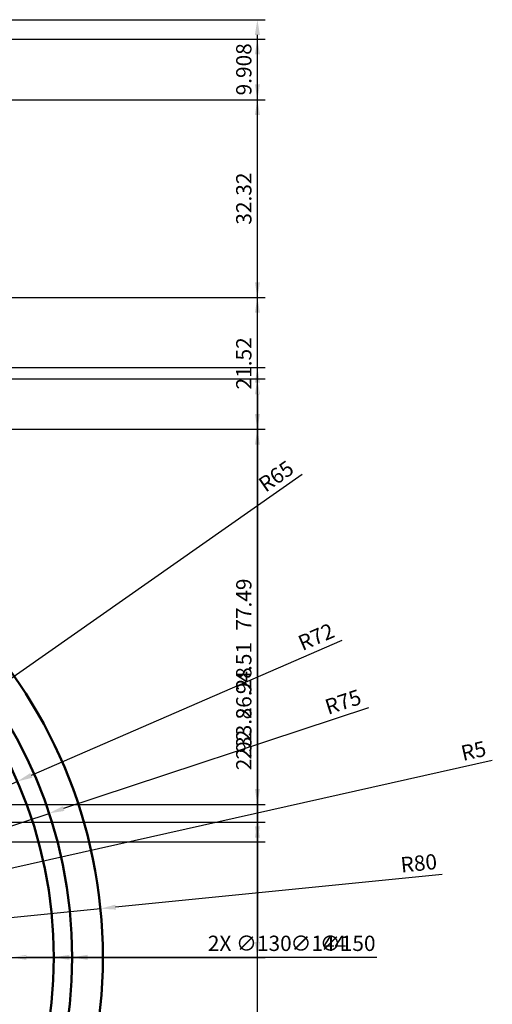
# Model space of a CAD drawing. Units: millimetres. Extents: x 1068 to 1546, y 1743 to 2032.
# Tile 9 of 9: x 1469 to 1546, y 1842 to 2003. Entities that reach past the tile are written whole.
import ezdxf

# ---------------------------------------------------------------- set-up
doc = ezdxf.new("R2010")
doc.units = ezdxf.units.MM
doc.layers.add('M-DIMS', color=2, linetype='Continuous', lineweight=25)
doc.layers.add('M-OUTL', color=7, linetype='Continuous', lineweight=50)
doc.styles.get("Standard").update_dxf_attribs({"font": 'arial.ttf'})
doc.dimstyles.new('ISO-25', dxfattribs={"dimtxt": 2.5, "dimasz": 2.5, "dimexe": 1.25, "dimexo": 0.625, "dimtad": 1, "dimtxsty": 'Standard', "dimcen": 2.5, "dimadec": 0, "dimazin": 0, "dimtfac": 1, "dimtmove": 0, "dimatfit": 3, "dimfxl": 1, "dimarcsym": 0})

# ---------------------------------------------------------------- blocks, each defined once
blk = doc.blocks.new('*D7')
at = {"layer": 'Defpoints', "color": 0, "transparency": 16777216}
for p in [(1407.11, 1850.85), (1402.23, 1849.76)]:
    blk.add_point(p, dxfattribs=at)
at = {"layer": 'M-DIMS', "color": 0, "lineweight": -2, "transparency": 16777216}
for p, q in [((1545.85, 1881.92), (1409.55, 1851.4)), ((1402.23, 1849.76), (1407.11, 1850.85))]:
    blk.add_line(p, q, dxfattribs=at)
at = {"layer": 'M-DIMS', "color": 0, "transparency": 16777216}
blk.add_solid([(1409.46, 1851.81), (1409.64, 1850.99), (1407.11, 1850.85)], dxfattribs=at)
at = {"layer": 'M-DIMS', "color": 0, "transparency": 16777216, "insert": (1542.85, 1883.19), "char_height": 2.5, "attachment_point": 5, "rotation": 12.6193}
blk.add_mtext('R5', dxfattribs=at)
blk = doc.blocks.new('*D8')
at = {"layer": 'Defpoints', "color": 0, "transparency": 16777216}
for p in [(1455.46, 1887.07), (1402.23, 1849.76)]:
    blk.add_point(p, dxfattribs=at)
at = {"layer": 'M-DIMS', "color": 0, "lineweight": -2, "transparency": 16777216}
for p, q in [((1514.78, 1928.64), (1457.51, 1888.5)), ((1402.23, 1849.76), (1455.46, 1887.07))]:
    blk.add_line(p, q, dxfattribs=at)
at = {"layer": 'M-DIMS', "color": 0, "transparency": 16777216}
blk.add_solid([(1457.27, 1888.84), (1457.75, 1888.16), (1455.46, 1887.07)], dxfattribs=at)
at = {"layer": 'M-DIMS', "color": 0, "transparency": 16777216, "insert": (1510.72, 1928.11), "char_height": 2.5, "attachment_point": 5, "rotation": 35.0221}
blk.add_mtext('R65', dxfattribs=at)
blk = doc.blocks.new('*D9')
at = {"layer": 'Defpoints', "color": 0, "transparency": 16777216}
for p in [(1468.25, 1878.49), (1402.23, 1849.76)]:
    blk.add_point(p, dxfattribs=at)
at = {"layer": 'M-DIMS', "color": 0, "lineweight": -2, "transparency": 16777216}
for p, q in [((1521.25, 1901.55), (1470.54, 1879.49)), ((1402.23, 1849.76), (1468.25, 1878.49))]:
    blk.add_line(p, q, dxfattribs=at)
at = {"layer": 'M-DIMS', "color": 0, "transparency": 16777216}
blk.add_solid([(1470.38, 1879.87), (1470.71, 1879.1), (1468.25, 1878.49)], dxfattribs=at)
at = {"layer": 'M-DIMS', "color": 0, "transparency": 16777216, "insert": (1517.2, 1901.84), "char_height": 2.5, "attachment_point": 5, "rotation": 23.5148}
blk.add_mtext('R72', dxfattribs=at)
blk = doc.blocks.new('*D10')
at = {"layer": 'Defpoints', "color": 0, "transparency": 16777216}
for p in [(1473.44, 1873.29), (1402.23, 1849.76)]:
    blk.add_point(p, dxfattribs=at)
at = {"layer": 'M-DIMS', "color": 0, "lineweight": -2, "transparency": 16777216}
for p, q in [((1525.61, 1890.52), (1475.82, 1874.07)), ((1402.23, 1849.76), (1473.44, 1873.29))]:
    blk.add_line(p, q, dxfattribs=at)
at = {"layer": 'M-DIMS', "color": 0, "transparency": 16777216}
blk.add_solid([(1475.69, 1874.47), (1475.95, 1873.68), (1473.44, 1873.29)], dxfattribs=at)
at = {"layer": 'M-DIMS', "color": 0, "transparency": 16777216, "insert": (1521.57, 1891.19), "char_height": 2.5, "attachment_point": 5, "rotation": 18.2811}
blk.add_mtext('R75', dxfattribs=at)
blk = doc.blocks.new('*D11')
at = {"layer": 'Defpoints', "color": 0, "transparency": 16777216}
for p in [(1481.83, 1857.72), (1402.23, 1849.76)]:
    blk.add_point(p, dxfattribs=at)
at = {"layer": 'M-DIMS', "color": 0, "lineweight": -2, "transparency": 16777216}
for p, q in [((1537.65, 1863.3), (1484.32, 1857.97)), ((1402.23, 1849.76), (1481.83, 1857.72))]:
    blk.add_line(p, q, dxfattribs=at)
at = {"layer": 'M-DIMS', "color": 0, "transparency": 16777216}
blk.add_solid([(1484.28, 1858.38), (1484.36, 1857.56), (1481.83, 1857.72)], dxfattribs=at)
at = {"layer": 'M-DIMS', "color": 0, "transparency": 16777216, "insert": (1533.87, 1864.83), "char_height": 2.5, "attachment_point": 5, "rotation": 5.7095}
blk.add_mtext('R80', dxfattribs=at)
blk = doc.blocks.new('*D25')
at = {"layer": 'Defpoints', "color": 0, "transparency": 16777216}
for p in [(1376.21, 2002.95), (1507.48, 2002.95), (1402.23, 1769.76)]:
    blk.add_point(p, dxfattribs=at)
at = {"layer": 'M-DIMS', "color": 0, "lineweight": -2, "transparency": 16777216}
for p, q in [((1376.84, 2002.95), (1508.73, 2002.95)), ((1507.48, 1772.26), (1507.48, 2000.45)), ((1402.85, 1769.76), (1508.73, 1769.76))]:
    blk.add_line(p, q, dxfattribs=at)
at = {"layer": 'M-DIMS', "color": 0, "transparency": 16777216}
for points in [[(1507.06, 2000.45), (1507.89, 2000.45), (1507.48, 2002.95)], [(1507.06, 1772.26), (1507.89, 1772.26), (1507.48, 1769.76)]]:
    blk.add_solid(points, dxfattribs=at)
at = {"layer": 'M-DIMS', "color": 0, "transparency": 16777216, "insert": (1505.58, 1886.35), "char_height": 2.5, "attachment_point": 5, "rotation": 90}
blk.add_mtext('233.2', dxfattribs=at)
blk = doc.blocks.new('*D27')
at = {"layer": 'Defpoints', "color": 0, "transparency": 16777216}
for p in [(1270.79, 1874.76), (1507.48, 1874.76), (1272.28, 1871.84)]:
    blk.add_point(p, dxfattribs=at)
at = {"layer": 'M-DIMS', "color": 0, "lineweight": -2, "transparency": 16777216}
for p, q in [((1507.48, 1877.26), (1507.48, 1887.52)), ((1271.41, 1874.76), (1508.73, 1874.76)), ((1507.48, 1871.84), (1507.48, 1874.76)), ((1272.9, 1871.84), (1508.73, 1871.84)), ((1507.48, 1869.34), (1507.48, 1866.84))]:
    blk.add_line(p, q, dxfattribs=at)
at = {"layer": 'M-DIMS', "color": 0, "transparency": 16777216}
for points in [[(1507.06, 1877.26), (1507.89, 1877.26), (1507.48, 1874.76)], [(1507.06, 1869.34), (1507.89, 1869.34), (1507.48, 1871.84)]]:
    blk.add_solid(points, dxfattribs=at)
at = {"layer": 'M-DIMS', "color": 0, "transparency": 16777216, "insert": (1505.58, 1883.64), "char_height": 2.5, "attachment_point": 5, "rotation": 90}
blk.add_mtext('2.92', dxfattribs=at)
blk = doc.blocks.new('*D34')
at = {"layer": 'Defpoints', "color": 0, "transparency": 16777216}
for p in [(1379.79, 1936.04), (1507.48, 1936.04), (1402.23, 1849.76)]:
    blk.add_point(p, dxfattribs=at)
at = {"layer": 'M-DIMS', "color": 0, "lineweight": -2, "transparency": 16777216}
for p, q in [((1380.41, 1936.04), (1508.73, 1936.04)), ((1507.48, 1852.26), (1507.48, 1933.54)), ((1402.85, 1849.76), (1508.73, 1849.76))]:
    blk.add_line(p, q, dxfattribs=at)
at = {"layer": 'M-DIMS', "color": 0, "transparency": 16777216}
for points in [[(1507.06, 1933.54), (1507.89, 1933.54), (1507.48, 1936.04)], [(1507.06, 1852.26), (1507.89, 1852.26), (1507.48, 1849.76)]]:
    blk.add_solid(points, dxfattribs=at)
at = {"layer": 'M-DIMS', "color": 0, "transparency": 16777216, "insert": (1505.58, 1892.9), "char_height": 2.5, "attachment_point": 5, "rotation": 90}
blk.add_mtext('86.28', dxfattribs=at)
blk = doc.blocks.new('*D35')
at = {"layer": 'Defpoints', "color": 0, "transparency": 16777216}
for p in [(1354.41, 1957.56), (1507.48, 1957.56), (1379.79, 1936.04)]:
    blk.add_point(p, dxfattribs=at)
at = {"layer": 'M-DIMS', "color": 0, "lineweight": -2, "transparency": 16777216}
for p, q in [((1355.03, 1957.56), (1508.73, 1957.56)), ((1507.48, 1938.54), (1507.48, 1955.06)), ((1380.41, 1936.04), (1508.73, 1936.04))]:
    blk.add_line(p, q, dxfattribs=at)
at = {"layer": 'M-DIMS', "color": 0, "transparency": 16777216}
for points in [[(1507.06, 1955.06), (1507.89, 1955.06), (1507.48, 1957.56)], [(1507.06, 1938.54), (1507.89, 1938.54), (1507.48, 1936.04)]]:
    blk.add_solid(points, dxfattribs=at)
at = {"layer": 'M-DIMS', "color": 0, "transparency": 16777216, "insert": (1505.58, 1946.8), "char_height": 2.5, "attachment_point": 5, "rotation": 90}
blk.add_mtext('21.52', dxfattribs=at)
blk = doc.blocks.new('*D36')
at = {"layer": 'Defpoints', "color": 0, "transparency": 16777216}
for p in [(1346.59, 1989.88), (1507.48, 1989.88), (1354.41, 1957.56)]:
    blk.add_point(p, dxfattribs=at)
at = {"layer": 'M-DIMS', "color": 0, "lineweight": -2, "transparency": 16777216}
for p, q in [((1347.22, 1989.88), (1508.73, 1989.88)), ((1507.48, 1960.06), (1507.48, 1987.38)), ((1355.03, 1957.56), (1508.73, 1957.56))]:
    blk.add_line(p, q, dxfattribs=at)
at = {"layer": 'M-DIMS', "color": 0, "transparency": 16777216}
for points in [[(1507.06, 1987.38), (1507.89, 1987.38), (1507.48, 1989.88)], [(1507.06, 1960.06), (1507.89, 1960.06), (1507.48, 1957.56)]]:
    blk.add_solid(points, dxfattribs=at)
at = {"layer": 'M-DIMS', "color": 0, "transparency": 16777216, "insert": (1505.58, 1973.72), "char_height": 2.5, "attachment_point": 5, "rotation": 90}
blk.add_mtext('32.32', dxfattribs=at)
blk = doc.blocks.new('*D37')
at = {"layer": 'Defpoints', "color": 0, "transparency": 16777216}
for p in [(1355.9, 1999.79), (1507.48, 1999.79), (1346.59, 1989.88)]:
    blk.add_point(p, dxfattribs=at)
at = {"layer": 'M-DIMS', "color": 0, "lineweight": -2, "transparency": 16777216}
for p, q in [((1356.52, 1999.79), (1508.73, 1999.79)), ((1507.48, 1992.38), (1507.48, 1997.29)), ((1347.22, 1989.88), (1508.73, 1989.88))]:
    blk.add_line(p, q, dxfattribs=at)
at = {"layer": 'M-DIMS', "color": 0, "transparency": 16777216}
for points in [[(1507.06, 1997.29), (1507.89, 1997.29), (1507.48, 1999.79)], [(1507.06, 1992.38), (1507.89, 1992.38), (1507.48, 1989.88)]]:
    blk.add_solid(points, dxfattribs=at)
at = {"layer": 'M-DIMS', "color": 0, "transparency": 16777216, "insert": (1505.58, 1994.84), "char_height": 2.5, "attachment_point": 5, "rotation": 90}
blk.add_mtext('9.908', dxfattribs=at)
blk = doc.blocks.new('*D48')
at = {"layer": 'Defpoints', "color": 0, "transparency": 16777216}
for p in [(1361.34, 1946.14), (1507.48, 1946.14), (1282.2, 1868.65)]:
    blk.add_point(p, dxfattribs=at)
at = {"layer": 'M-DIMS', "color": 0, "lineweight": -2, "transparency": 16777216}
for p, q in [((1361.96, 1946.14), (1508.73, 1946.14)), ((1507.48, 1871.15), (1507.48, 1943.64)), ((1282.82, 1868.65), (1508.73, 1868.65))]:
    blk.add_line(p, q, dxfattribs=at)
at = {"layer": 'M-DIMS', "color": 0, "transparency": 16777216}
for points in [[(1507.06, 1943.64), (1507.89, 1943.64), (1507.48, 1946.14)], [(1507.06, 1871.15), (1507.89, 1871.15), (1507.48, 1868.65)]]:
    blk.add_solid(points, dxfattribs=at)
at = {"layer": 'M-DIMS', "color": 0, "transparency": 16777216, "insert": (1505.58, 1907.39), "char_height": 2.5, "attachment_point": 5, "rotation": 90}
blk.add_mtext('77.49', dxfattribs=at)
blk = doc.blocks.new('*D52')
at = {"layer": 'Defpoints', "color": 0, "transparency": 16777216}
for p in [(1372.84, 1944.27), (1402.23, 1849.76), (1507.48, 1849.76)]:
    blk.add_point(p, dxfattribs=at)
at = {"layer": 'M-DIMS', "color": 0, "lineweight": -2, "transparency": 16777216}
for p, q in [((1373.47, 1944.27), (1508.73, 1944.27)), ((1507.48, 1941.77), (1507.48, 1852.26)), ((1402.85, 1849.76), (1508.73, 1849.76))]:
    blk.add_line(p, q, dxfattribs=at)
at = {"layer": 'M-DIMS', "color": 0, "transparency": 16777216}
for points in [[(1507.06, 1941.77), (1507.89, 1941.77), (1507.48, 1944.27)], [(1507.06, 1852.26), (1507.89, 1852.26), (1507.48, 1849.76)]]:
    blk.add_solid(points, dxfattribs=at)
at = {"layer": 'M-DIMS', "color": 0, "transparency": 16777216, "insert": (1505.58, 1897.02), "char_height": 2.5, "attachment_point": 5, "rotation": 90}
blk.add_mtext('94.51', dxfattribs=at)
blk = doc.blocks.new('*D53')
at = {"layer": 'Defpoints', "color": 0, "transparency": 16777216}
for p in [(1332.93, 1889.74), (1471.52, 1809.79)]:
    blk.add_point(p, dxfattribs=at)
at = {"layer": 'M-DIMS', "color": 0, "lineweight": -2, "transparency": 16777216}
for p, q in [((1330.77, 1890.99), (1328.6, 1892.24)), ((1332.93, 1889.74), (1471.52, 1809.79)), ((1517.21, 1783.43), (1473.69, 1808.54))]:
    blk.add_line(p, q, dxfattribs=at)
at = {"layer": 'M-DIMS', "color": 0, "transparency": 16777216}
for points in [[(1330.98, 1891.35), (1330.56, 1890.63), (1332.93, 1889.74)], [(1473.9, 1808.9), (1473.48, 1808.18), (1471.52, 1809.79)]]:
    blk.add_solid(points, dxfattribs=at)
at = {"layer": 'M-DIMS', "color": 0, "transparency": 16777216, "insert": (1514.09, 1787.51), "char_height": 2.5, "attachment_point": 5, "rotation": 330.0197}
blk.add_mtext('∅160', dxfattribs=at)
blk = doc.blocks.new('*D54')
at = {"layer": 'Defpoints', "color": 0, "transparency": 16777216}
for p in [(1327.23, 1849.76), (1477.23, 1849.76)]:
    blk.add_point(p, dxfattribs=at)
at = {"layer": 'M-DIMS', "color": 0, "lineweight": -2, "transparency": 16777216}
for p, q in [((1324.73, 1849.76), (1322.23, 1849.76)), ((1327.23, 1849.76), (1477.23, 1849.76)), ((1526.97, 1849.76), (1479.73, 1849.76))]:
    blk.add_line(p, q, dxfattribs=at)
at = {"layer": 'M-DIMS', "color": 0, "transparency": 16777216}
for points in [[(1324.73, 1850.18), (1324.73, 1849.35), (1327.23, 1849.76)], [(1479.73, 1850.18), (1479.73, 1849.35), (1477.23, 1849.76)]]:
    blk.add_solid(points, dxfattribs=at)
at = {"layer": 'M-DIMS', "color": 0, "transparency": 16777216, "insert": (1522.23, 1851.73), "char_height": 2.5, "attachment_point": 5, "rotation": 359.9998}
blk.add_mtext('∅150', dxfattribs=at)
blk = doc.blocks.new('*D55')
at = {"layer": 'Defpoints', "color": 0, "transparency": 16777216}
for p in [(1330.23, 1849.76), (1474.23, 1849.76)]:
    blk.add_point(p, dxfattribs=at)
at = {"layer": 'M-DIMS', "color": 0, "lineweight": -2, "transparency": 16777216}
for p, q in [((1327.73, 1849.76), (1325.23, 1849.76)), ((1330.23, 1849.76), (1474.23, 1849.76)), ((1522.17, 1849.76), (1476.73, 1849.76))]:
    blk.add_line(p, q, dxfattribs=at)
at = {"layer": 'M-DIMS', "color": 0, "transparency": 16777216}
for points in [[(1327.73, 1850.18), (1327.73, 1849.35), (1330.23, 1849.76)], [(1476.73, 1850.18), (1476.73, 1849.35), (1474.23, 1849.76)]]:
    blk.add_solid(points, dxfattribs=at)
at = {"layer": 'M-DIMS', "color": 0, "transparency": 16777216, "insert": (1517.43, 1851.73), "char_height": 2.5, "attachment_point": 5, "rotation": 359.9997}
blk.add_mtext('∅144', dxfattribs=at)
blk = doc.blocks.new('*D56')
at = {"layer": 'Defpoints', "color": 0, "transparency": 16777216}
for p in [(1337.23, 1849.76), (1467.23, 1849.76)]:
    blk.add_point(p, dxfattribs=at)
at = {"layer": 'M-DIMS', "color": 0, "lineweight": -2, "transparency": 16777216}
for p, q in [((1334.73, 1849.76), (1332.23, 1849.76)), ((1337.23, 1849.76), (1467.23, 1849.76)), ((1513.61, 1849.76), (1469.73, 1849.76))]:
    blk.add_line(p, q, dxfattribs=at)
at = {"layer": 'M-DIMS', "color": 0, "transparency": 16777216}
for points in [[(1334.73, 1850.18), (1334.73, 1849.35), (1337.23, 1849.76)], [(1469.73, 1850.18), (1469.73, 1849.35), (1467.23, 1849.76)]]:
    blk.add_solid(points, dxfattribs=at)
at = {"layer": 'M-DIMS', "color": 0, "transparency": 16777216, "insert": (1506.23, 1851.73), "char_height": 2.5, "attachment_point": 5, "rotation": 359.9997}
blk.add_mtext('2X ∅130', dxfattribs=at)

msp = doc.modelspace()

# ---------------------------------------------------------------- linework, layer by layer
at = {"layer": 'M-OUTL'}
for radius in [80, 75, 72]:
    msp.add_circle((1402.2281, 1849.7623), radius, dxfattribs=at)

# ---------------------------------------------------------------- dimensions: what is measured, and where the dimension line sits
at = {"layer": 'M-DIMS'}
for base, p1, p2, override, picture, middle in [((1507.4781, 2002.9476), (1402.2281, 1769.7623), (1376.2106, 2002.9476), {"dimdec": 1, "dimlfac": 1, "dimrnd": 0, "dimzin": 0, "dimdsep": 46, "dimlunit": 2}, '*D25', (1505.5758, 1886.355)), ((1507.4781, 1999.7899), (1346.5904, 1989.8822), (1355.8981, 1999.7899), {"dimdec": 3, "dimlfac": 1, "dimrnd": 0, "dimzin": 0, "dimdsep": 46, "dimlunit": 2}, '*D37', (1505.5767, 1994.836)), ((1507.4781, 1989.8822), (1354.405, 1957.5607), (1346.5904, 1989.8822), {"dimdec": 2, "dimlfac": 1, "dimrnd": 0, "dimzin": 0, "dimdsep": 46, "dimlunit": 2}, '*D36', (1505.5758, 1973.7215)), ((1507.4781, 1957.5607), (1379.7864, 1936.0393), (1354.405, 1957.5607), {"dimdec": 2, "dimlfac": 1, "dimrnd": 0, "dimzin": 0, "dimdsep": 46, "dimlunit": 2}, '*D35', (1505.5767, 1946.8)), ((1507.4781, 1946.1377), (1282.1954, 1868.6519), (1361.339, 1946.1377), {"dimdec": 2, "dimlfac": 1, "dimrnd": 0, "dimzin": 0, "dimdsep": 46, "dimlunit": 2}, '*D48', (1505.5767, 1907.3948)), ((1507.4781, 1849.7623), (1372.8438, 1944.2719), (1402.2281, 1849.7623), {"dimdec": 2, "dimlfac": 1, "dimrnd": 0, "dimzin": 0, "dimdsep": 46, "dimlunit": 2}, '*D52', (1505.5767, 1897.0171)), ((1507.4781, 1936.0393), (1402.2281, 1849.7623), (1379.7864, 1936.0393), {"dimdec": 2, "dimlfac": 1, "dimrnd": 0, "dimzin": 0, "dimdsep": 46, "dimlunit": 2}, '*D34', (1505.5767, 1892.9008)), ((1507.4781, 1874.7623), (1272.2751, 1871.8409), (1270.787, 1874.7623), {"dimdec": 2, "dimlfac": 1, "dimrnd": 0, "dimzin": 0, "dimdsep": 46, "dimlunit": 2}, '*D27', (1505.5767, 1883.6428))]:
    dim = msp.add_linear_dim(base=base, p1=p1, p2=p2, angle=90, dimstyle='ISO-25', override=override, dxfattribs=at)
    dim.commit()
    dim.dimension.update_dxf_attribs({"geometry": picture, "text_midpoint": middle})
for mpoint, picture, middle in [((1455.4586, 1887.0653), '*D8', (1511.8133, 1926.5577)), ((1468.249, 1878.4894), '*D9', (1517.9503, 1900.1154)), ((1473.4428, 1873.2883), '*D10', (1522.1694, 1889.3852)), ((1407.1073, 1850.8547), '*D7', (1543.265, 1881.3376)), ((1481.8313, 1857.7211), '*D11', (1534.0596, 1862.943))]:
    dim = msp.add_radius_dim(center=(1402.2281, 1849.7623), mpoint=mpoint, dimstyle='ISO-25', override={"dimclrd": 0, "dimclre": 0, "dimclrt": 0}, dxfattribs=at)
    dim.commit()
    dim.dimension.update_dxf_attribs({"geometry": picture, "text_midpoint": middle, "dimtype": 164})
for p1, p2, picture, middle in [((1332.9323, 1889.7385), (1471.5239, 1809.7862), '*D53', (1513.1014, 1785.8005)), ((1327.2281, 1849.7627), (1477.2281, 1849.762), '*D54', (1522.2281, 1849.7618)), ((1330.2281, 1849.7627), (1474.2281, 1849.762), '*D55', (1517.4281, 1849.7618))]:
    dim = msp.add_diameter_dim_2p(p1=p1, p2=p2, dimstyle='ISO-25', override={"dimdec": 0, "dimlfac": 1, "dimrnd": 0, "dimzin": 0, "dimdsep": 46, "dimlunit": 2}, dxfattribs=at)
    dim.commit()
    dim.dimension.update_dxf_attribs({"geometry": picture, "text_midpoint": middle, "dimtype": 163})
dim = msp.add_diameter_dim_2p(p1=(1337.2281, 1849.7627), p2=(1467.2281, 1849.762), text='2X <>', dimstyle='ISO-25', override={"dimdec": 0, "dimlfac": 1, "dimrnd": 0, "dimzin": 0, "dimdsep": 46, "dimlunit": 2}, dxfattribs=at)
dim.commit()
dim.dimension.update_dxf_attribs({"geometry": '*D56', "text_midpoint": (1506.2281, 1849.7618), "dimtype": 163})

doc.saveas('drawing.dxf')
